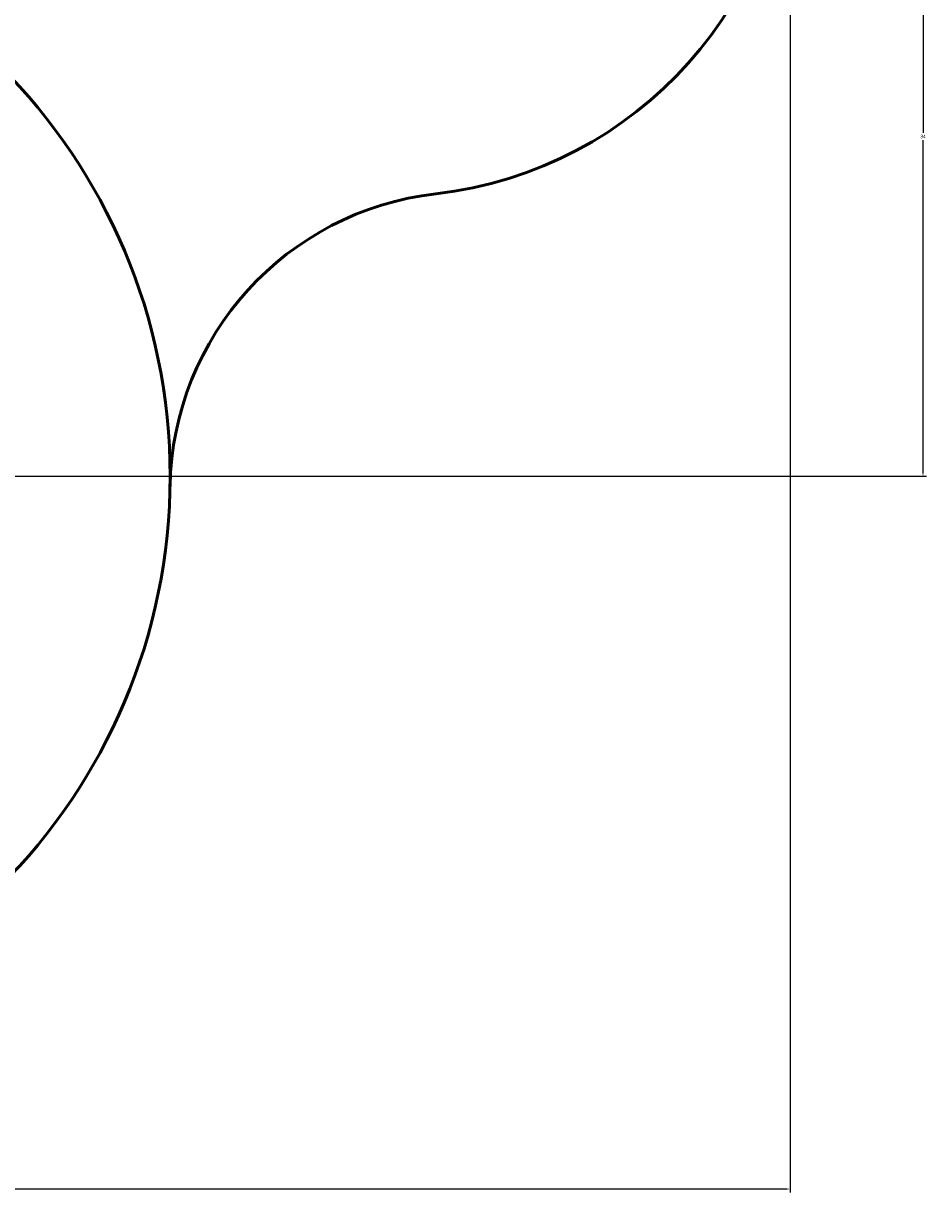
# Model space of a CAD drawing. Units: inches. Extents: x -11 to 126, y -62 to 82.
# Tile 5 of 10: x 81 to 126, y -57 to 1. Entities that reach past the tile are written whole.
import ezdxf

# ---------------------------------------------------------------- set-up
doc = ezdxf.new("R2010")
doc.units = ezdxf.units.IN
doc.header["$MEASUREMENT"] = 0
doc.layers.add('M-DIMS', color=2, linetype='Continuous', lineweight=18)
doc.layers.add('M-OUTL', color=7, linetype='Continuous', lineweight=50)
doc.styles.get("Standard").update_dxf_attribs({"font": 'arial.ttf'})
doc.dimstyles.get("Standard").update_dxf_attribs({"dimtxt": 0.18, "dimasz": 0.18, "dimexe": 0.18, "dimexo": 0.0625, "dimgap": 0.09, "dimtad": 0, "dimtih": 1, "dimtoh": 1, "dimdec": 4, "dimzin": 0, "dimdsep": 46, "dimtxsty": 'Standard', "dimcen": 0.09, "dimadec": 0, "dimazin": 0, "dimtfac": 1, "dimtdec": 4, "dimtofl": 0, "dimtmove": 0, "dimatfit": 3, "dimfxl": 1, "dimtolj": 1, "dimtzin": 0, "dimarcsym": 0})

# ---------------------------------------------------------------- blocks, each defined once
blk = doc.blocks.new('*D5')
at = {"layer": 'Defpoints', "color": 0, "transparency": 16777216}
for p in [(119.232, 12.354), (-0.749, 11.479), (119.232, -57.296)]:
    blk.add_point(p, dxfattribs=at)
at = {"layer": 'M-DIMS', "color": 0, "lineweight": -2, "transparency": 16777216}
for p, q in [((119.232, 12.292), (119.232, -57.476)), ((-0.749, 11.416), (-0.749, -57.476)), ((-0.569, -57.296), (58.786, -57.296)), ((119.052, -57.296), (59.696, -57.296))]:
    blk.add_line(p, q, dxfattribs=at)
at = {"layer": 'M-DIMS', "color": 0, "transparency": 16777216}
for points in [[(-0.569, -57.266), (-0.569, -57.326), (-0.749, -57.296)], [(119.052, -57.266), (119.052, -57.326), (119.232, -57.296)]]:
    blk.add_solid(points, dxfattribs=at)
at = {"layer": 'M-DIMS', "color": 0, "transparency": 16777216, "insert": (59.241, -57.296), "char_height": 0.18, "attachment_point": 5}
blk.add_mtext('\\A1;119.98', dxfattribs=at)
blk = doc.blocks.new('*D9')
at = {"layer": 'Defpoints', "color": 0, "transparency": 16777216}
for p in [(99.232, 12.354), (125.882, 12.354), (59.232, -21.646)]:
    blk.add_point(p, dxfattribs=at)
at = {"layer": 'M-DIMS', "color": 0, "lineweight": -2, "transparency": 16777216}
for p, q in [((99.294, 12.354), (126.062, 12.354)), ((125.882, 12.174), (125.882, -4.464)), ((125.882, -21.466), (125.882, -4.828)), ((59.294, -21.646), (126.062, -21.646))]:
    blk.add_line(p, q, dxfattribs=at)
at = {"layer": 'M-DIMS', "color": 0, "transparency": 16777216}
for points in [[(125.852, 12.174), (125.912, 12.174), (125.882, 12.354)], [(125.852, -21.466), (125.912, -21.466), (125.882, -21.646)]]:
    blk.add_solid(points, dxfattribs=at)
at = {"layer": 'M-DIMS', "color": 0, "transparency": 16777216, "insert": (125.882, -4.646), "char_height": 0.18, "attachment_point": 5}
blk.add_mtext('\\A1;34', dxfattribs=at)

msp = doc.modelspace()

# ---------------------------------------------------------------- linework, layer by layer
at = {"layer": 'M-OUTL'}
msp.add_circle((59.232, -21.646), 29, dxfattribs=at)
for centre, radius, start, end in [((99.232, 12.354), 20, 276.55128, 83.44872), ((103.225, -22.417), 15, 96.55128, 178.99538)]:
    msp.add_arc(centre, radius, start, end, dxfattribs=at)

# ---------------------------------------------------------------- dimensions: what is measured, and where the dimension line sits
at = {"layer": 'M-DIMS'}
dim = msp.add_linear_dim(base=(119.232, -57.296), p1=(-0.749, 11.479), p2=(119.232, 12.354), dimstyle='Standard', override={"dimdec": 2, "dimlfac": 1, "dimrnd": 0, "dimzin": 0, "dimdsep": 46, "dimlunit": 2}, dxfattribs=at)
dim.commit()
dim.dimension.update_dxf_attribs({"geometry": '*D5', "text_midpoint": (59.241, -57.296)})
dim = msp.add_linear_dim(base=(125.882, 12.354), p1=(59.232, -21.646), p2=(99.232, 12.354), angle=90, dimstyle='Standard', override={"dimdec": 0, "dimlfac": 1, "dimrnd": 0, "dimzin": 0, "dimdsep": 46, "dimlunit": 2}, dxfattribs=at)
dim.commit()
dim.dimension.update_dxf_attribs({"geometry": '*D9', "text_midpoint": (125.882, -4.646)})

doc.saveas('drawing.dxf')
